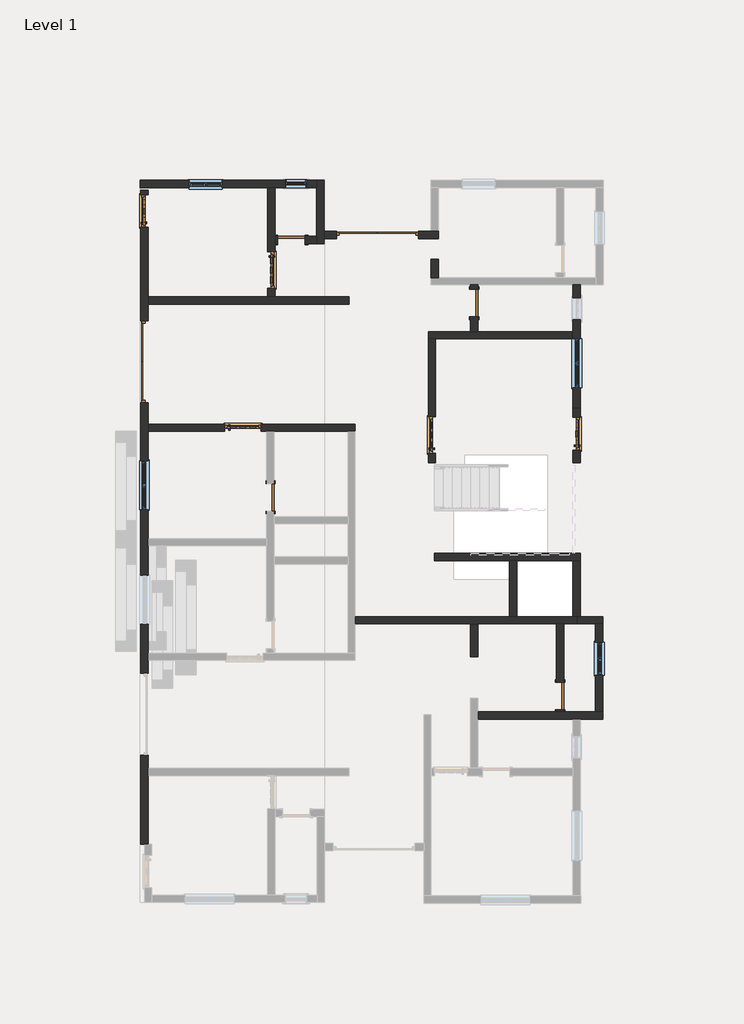
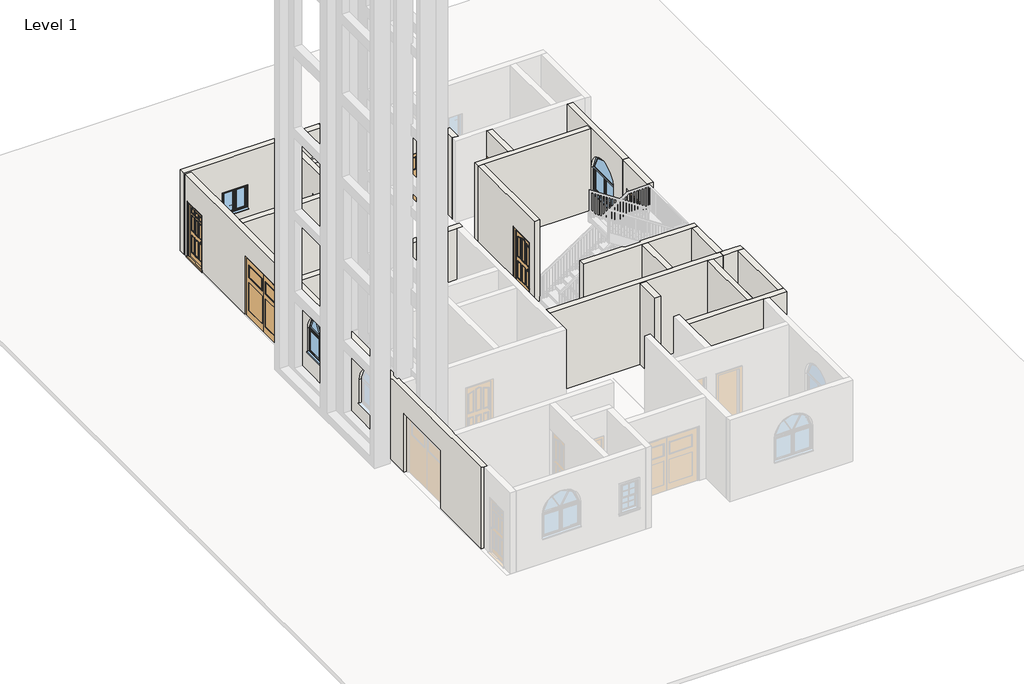
# One storey, part 2 of 4: 23 walls, 11 doors, 5 windows.
"""IFC4 building model written with IfcOpenShell, lengths in millimetres."""

from ifc_helpers import new_model, si_unit, point, frame, frame_2d, origin, origin_with_axes, place, context, project, spatial, polyline, circle_curve, trimmed, segment, composite_curve, outline, extrude, faceted_brep, transform, mapped, element, save
from ifc_brep_helpers import plane_surface, revolved_surface, advanced_brep
from components import doors_extsgl_5_910x2110mm_99758a98, doors_extsgl_5_910x2110mm_d3ca6061, doors_extsgl_6_1010x2110mm_b93c615f, doors_extsgl_6_1010x2110mm_efbaf1af, doors_garage_timber_side_hung_glazing_2270x2050mm_ae99176d, doors_garage_timber_side_hung_glazing_2270x2200mm_badb7014, door_fadea3f2, door_53b1b562, window_679d2811, windows_arched_1360x910mm_c5754810, windows_dbl_w_glazing_bars_910x910mm_41eba874

model = new_model("IFC4")

# Units and contexts
model_context = context("Model", 3, world=origin())
ifc_project = project(units=[si_unit("LENGTHUNIT", "METRE", prefix="MILLI")], contexts=[model_context])

# Site, building, storey
site = spatial("IfcSite", under=ifc_project)
building = spatial("IfcBuilding", under=site)
storey = spatial("IfcBuildingStorey", under=building, Name="Level 1", Elevation=0.0)

# Doors
placement = place(None, origin())
doors_extsgl_5_910x2110mm_shape = doors_extsgl_5_910x2110mm_99758a98(model_context)
element("IfcDoor", 1, ObjectType="Doors_ExtSgl_5 : 910x2110mm", at=placement, inside=storey, context=model_context, shape_type="MappedRepresentation", body=[
    mapped(doors_extsgl_5_910x2110mm_shape, transform((5761.5890963, 2376.5107951, 0.0), x_axis=(0.0, 1.0, 0.0), y_axis=(-1.0, 0.0, 0.0), z_axis=(0.0, 0.0, 1.0))),
])
doors_extsgl_5_910x2110mm_2_shape = doors_extsgl_5_910x2110mm_d3ca6061(model_context)
element("IfcDoor", 2, ObjectType="Doors_ExtSgl_5 : 910x2110mm", at=placement, inside=storey, context=model_context, shape_type="MappedRepresentation", body=[
    mapped(doors_extsgl_5_910x2110mm_2_shape, transform((-6229.2013636, 8553.74399, 0.0), x_axis=(0.0, 1.0, 0.0), y_axis=(-1.0, 0.0, 0.0), z_axis=(0.0, 0.0, 1.0))),
])
doors_extsgl_6_1010x2110mm_shape = doors_extsgl_6_1010x2110mm_b93c615f(model_context)
doors_extsgl_6_1010x2110mm_2_shape = doors_extsgl_6_1010x2110mm_efbaf1af(model_context)
element("IfcDoor", 3, ObjectType="Doors_ExtSgl_6 : 1010x2110mm", at=placement, inside=storey, context=model_context, shape_type="MappedRepresentation", body=[
    mapped(doors_extsgl_6_1010x2110mm_shape, transform((-2709.3109037, 6913.1295584, 0.0), x_axis=(0.0, -1.0, 0.0), y_axis=(1.0, 0.0, 0.0), z_axis=(0.0, 0.0, 1.0))),
    mapped(doors_extsgl_6_1010x2110mm_2_shape, transform((-2709.3109037, 6913.1295584, 0.0), x_axis=(0.0, -1.0, 0.0), y_axis=(1.0, 0.0, 0.0), z_axis=(0.0, 0.0, 1.0))),
])
element("IfcDoor", 4, ObjectType="Doors_ExtSgl_6 : 1010x2110mm", at=placement, inside=storey, context=model_context, shape_type="MappedRepresentation", body=[
    mapped(doors_extsgl_6_1010x2110mm_shape, transform((1748.3890963, 2341.0628918, 0.0), x_axis=(0.0, 1.0, 0.0), y_axis=(-1.0, 0.0, 0.0), z_axis=(0.0, 0.0, 1.0))),
    mapped(doors_extsgl_6_1010x2110mm_2_shape, transform((1748.3890963, 2341.0628918, 0.0), x_axis=(0.0, 1.0, 0.0), y_axis=(-1.0, 0.0, 0.0), z_axis=(0.0, 0.0, 1.0))),
])
element("IfcDoor", 5, ObjectType="Doors_ExtSgl_6 : 1010x2110mm", at=placement, inside=storey, context=model_context, shape_type="MappedRepresentation", body=[
    mapped(doors_extsgl_6_1010x2110mm_shape, transform((-3496.7442371, 2544.2962251, 0.0), x_axis=(1.0, 0.0, 0.0), y_axis=(0.0, 1.0, 0.0), z_axis=(0.0, 0.0, 1.0))),
    mapped(doors_extsgl_6_1010x2110mm_2_shape, transform((-3496.7442371, 2544.2962251, 0.0), x_axis=(1.0, 0.0, 0.0), y_axis=(0.0, 1.0, 0.0), z_axis=(0.0, 0.0, 1.0))),
])
doors_garage_timber_side_hung_glazing_2270x2050mm_shape = doors_garage_timber_side_hung_glazing_2270x2050mm_ae99176d(model_context)
element("IfcDoor", 6, ObjectType="Doors_Garage_Timber_Side_Hung_Glazing : 2270x2050mm", at=placement, inside=storey, context=model_context, shape_type="MappedRepresentation", body=[
    mapped(doors_garage_timber_side_hung_glazing_2270x2050mm_shape, transform((237.0890963, 7890.9962251, 0.0), x_axis=(1.0, 0.0, 0.0), y_axis=(0.0, 1.0, 0.0), z_axis=(0.0, 0.0, 1.0))),
])
doors_garage_timber_side_hung_glazing_2270x2200mm_shape = doors_garage_timber_side_hung_glazing_2270x2200mm_badb7014(model_context)
element("IfcDoor", 7, ObjectType="Doors_Garage_Timber_Side_Hung_Glazing : 2270x2200mm", at=placement, inside=storey, context=model_context, shape_type="MappedRepresentation", body=[
    mapped(doors_garage_timber_side_hung_glazing_2270x2200mm_shape, transform((-6229.2013636, 4373.0962251, 0.0), x_axis=(0.0, -1.0, 0.0), y_axis=(1.0, 0.0, 0.0), z_axis=(0.0, 0.0, 1.0))),
])
door_shape = door_fadea3f2(model_context)
element("IfcDoor", 8, ObjectType="Single-Flush : 30\" x 80\"", at=placement, inside=storey, context=model_context, shape_type="MappedRepresentation", body=[
    mapped(door_shape, transform((5304.3890963, -4897.9037749, 0.0), x_axis=(0.0, -1.0, 0.0), y_axis=(1.0, 0.0, 0.0), z_axis=(0.0, 0.0, 1.0))),
])
door_2_shape = door_53b1b562(model_context)
element("IfcDoor", 9, ObjectType="Single-Flush : 30\" x 80\"", at=placement, inside=storey, context=model_context, shape_type="MappedRepresentation", body=[
    mapped(door_2_shape, transform((-2150.5109037, 7751.2962251, 0.0), x_axis=(-1.0, 0.0, 0.0), y_axis=(0.0, -1.0, 0.0), z_axis=(0.0, 0.0, 1.0))),
])
element("IfcDoor", 10, ObjectType="Single-Flush : 30\" x 80\"", at=placement, inside=storey, context=model_context, shape_type="MappedRepresentation", body=[
    mapped(door_2_shape, transform((2916.7890963, 5998.6962251, 0.0), x_axis=(0.0, 1.0, 0.0), y_axis=(-1.0, 0.0, 0.0), z_axis=(0.0, 0.0, 1.0))),
])
element("IfcDoor", 11, ObjectType="Single-Flush : 30\" x 80\"", at=placement, inside=storey, context=model_context, shape_type="MappedRepresentation", body=[
    mapped(door_2_shape, transform((-2734.7109037, 613.8962251, 0.0), x_axis=(0.0, 1.0, 0.0), y_axis=(-1.0, 0.0, 0.0), z_axis=(0.0, 0.0, 1.0))),
])

# Walls
element("IfcWall", 12, ObjectType="Generic - 9\" w", at=placement, inside=storey, context=model_context, shape_type="SweptSolid", body=[
    extrude(outline(polyline([(6506.6962251, 0.0), (3087.7441284, 0.0), (3087.7441284, 3048.0), (6506.6962251, 3048.0), (6506.6962251, 0.0)]), holes=[polyline([(6151.0962251, 1981.2), (5541.4962251, 1981.2), (5541.4962251, 914.4), (6151.0962251, 914.4), (6151.0962251, 1981.2)]), composite_curve([segment(polyline([(5016.7786331, 685.6617803), (5016.7786331, 1595.6617803)]), True, "CONTINUOUS"), segment(trimmed(circle_curve(frame_2d((4336.7786331, 1595.6617803)), 680.0), [point((5016.7786331, 1595.6617803))], [point((3656.7786331, 1595.6617803))], True, "CARTESIAN"), True, "CONTINUOUS"), segment(polyline([(3656.7786331, 1595.6617803), (3656.7786331, 685.6617803), (5016.7786331, 685.6617803)]), True, "CONTINUOUS")], self_intersect=False)]), frame((5659.9890963, 0.0, 0.0), z_axis=(1.0, 0.0, 0.0), x_axis=(0.0, 1.0, 0.0)), (0.0, 0.0, 1.0), 203.2),
])
element("IfcWall", 13, ObjectType="Generic - 9\" w", at=placement, inside=storey, context=model_context, shape_type="Brep", body=[
    faceted_brep([(6485.4890963, -2688.1037749, 0.0), (5863.1890963, -2688.1037749, 0.0), (5761.5890963, -2688.1037749, 0.0), (5761.5890963, -2688.1037749, 3048.0), (5863.1890963, -2688.1037749, 3048.0), (6485.4890963, -2688.1037749, 3048.0), (6485.4890963, -2891.3037749, 0.0), (6485.4890963, -2891.3037749, 3048.0), (6282.2890963, -2891.3037749, 3048.0), (5761.5890963, -2891.3037749, 3048.0), (5761.5890963, -2891.3037749, 0.0), (6282.2890963, -2891.3037749, 0.0)], [[[0, 1, 2, 3, 4, 5]], [[6, 7, 8, 9, 10, 11]], [[2, 1, 0, 6, 11, 10]], [[3, 2, 10, 9]], [[5, 4, 3, 9, 8, 7]], [[0, 5, 7, 6]]]),
])
element("IfcWall", 14, ObjectType="Generic - 9\" w", at=placement, inside=storey, context=model_context, shape_type="Brep", body=[
    faceted_brep([(5761.5890963, -2688.1037749, 0.0), (5659.9890963, -2688.1037749, 0.0), (4097.8890963, -2688.1037749, 0.0), (3894.6890963, -2688.1037749, 0.0), (-385.2109037, -2688.1037749, 0.0), (-385.2109037, -2688.1037749, 3048.0), (3894.6890963, -2688.1037749, 3048.0), (4097.8890963, -2688.1037749, 3048.0), (5659.9890963, -2688.1037749, 3048.0), (5761.5890963, -2688.1037749, 3048.0), (5761.5890963, -2891.3037749, 0.0), (5761.5890963, -2891.3037749, 3048.0), (5405.9890963, -2891.3037749, 3048.0), (5202.7890963, -2891.3037749, 3048.0), (-385.2109037, -2891.3037749, 3048.0), (-385.2109037, -2891.3037749, 0.0), (5202.7890963, -2891.3037749, 0.0), (5405.9890963, -2891.3037749, 0.0)], [[[0, 1, 2, 3, 4, 5, 6, 7, 8, 9]], [[10, 11, 12, 13, 14, 15, 16, 17]], [[4, 3, 2, 1, 0, 10, 17, 16, 15]], [[9, 8, 7, 6, 5, 14, 13, 12, 11]], [[0, 9, 11, 10]], [[5, 4, 15, 14]]]),
])
element("IfcWall", 15, ObjectType="Generic - 9\" w", at=placement, inside=storey, context=model_context, shape_type="SweptSolid", body=[
    extrude(outline(polyline([(3894.6890963, -2688.1037749), (3894.6890963, -1138.7037749), (4097.8890963, -1138.7037749), (4097.8890963, -2688.1037749), (3894.6890963, -2688.1037749)])), origin_with_axes(), (0.0, 0.0, 1.0), 3048.0),
])
element("IfcWall", 16, ObjectType="Generic - 9\" w", at=placement, inside=storey, context=model_context, shape_type="Brep", body=[
    faceted_brep([(5863.1890963, -935.5037749, 0.0), (1812.4805171, -935.5037749, 0.0), (1812.4805171, -935.5037749, 3048.0), (5863.1890963, -935.5037749, 3048.0), (5863.1890963, -1138.7037749, 0.0), (5863.1890963, -1138.7037749, 3048.0), (5659.9890963, -1138.7037749, 3048.0), (4097.8890963, -1138.7037749, 3048.0), (3894.6890963, -1138.7037749, 3048.0), (1812.4805171, -1138.7037749, 3048.0), (1812.4805171, -1138.7037749, 0.0), (3894.6890963, -1138.7037749, 0.0), (4097.8890963, -1138.7037749, 0.0), (5659.9890963, -1138.7037749, 0.0)], [[[0, 1, 2, 3]], [[4, 5, 6, 7, 8, 9, 10, 11, 12, 13]], [[1, 0, 4, 13, 12, 11, 10]], [[2, 1, 10, 9]], [[3, 2, 9, 8, 7, 6, 5]], [[0, 3, 5, 4]]]),
])
element("IfcWall", 17, ObjectType="Generic - 9\" w", at=placement, inside=storey, context=model_context, shape_type="Brep", body=[
    faceted_brep([(5659.9890963, -1138.7037749, 0.0), (5659.9890963, -2688.1037749, 0.0), (5659.9890963, -2688.1037749, 3048.0), (5659.9890963, -1138.7037749, 3048.0), (5863.1890963, -1138.7037749, 0.0), (5863.1890963, -1138.7037749, 3048.0), (5863.1890963, -2688.1037749, 3048.0), (5863.1890963, -2688.1037749, 0.0), (5761.5890963, -2688.1037749, 0.0), (5761.5890963, -2688.1037749, 3048.0)], [[[0, 1, 2, 3]], [[4, 5, 6, 7]], [[1, 0, 4, 7, 8]], [[3, 2, 9, 6, 5]], [[2, 1, 8, 7, 6, 9]], [[0, 3, 5, 4]]]),
])
element("IfcWall", 18, ObjectType="Generic - 9\" w", at=placement, inside=storey, context=model_context, shape_type="AdvancedBrep", body=[
    advanced_brep(
    [(-6330.8013636, 3238.0962251, 0.0), (-6330.8013636, -4267.1251987, 0.0), (-6330.8013636, -4267.1251987, 2200.0), (-6330.8013636, -6537.1251987, 2200.0), (-6330.8013636, -6537.1251987, 0.0), (-6330.8013636, -9007.7845215, 0.0), (-6330.8013636, -9007.7845215, 3048.0), (-6330.8013636, 9129.8816143, 3048.0), (-6330.8013636, 9129.8816143, 0.0), (-6330.8013636, 9008.7773233, 0.0), (-6330.8013636, 9008.7773233, 2110.0), (-6330.8013636, 8098.7773233, 2110.0), (-6330.8013636, 8098.7773233, 0.0), (-6330.8013636, 5508.0962251, 0.0), (-6330.8013636, 5508.0962251, 2200.0), (-6330.8013636, 3238.0962251, 2200.0), (-6330.8013636, 276.7962251, 914.4), (-6330.8013636, 1636.7962251, 914.4), (-6330.8013636, 1636.7962251, 1824.4), (-6330.8013636, 276.7962251, 1824.4), (-6330.8013636, -1538.2037749, 914.4), (-6330.8013636, -1538.2037749, 1824.4), (-6330.8013636, -2898.2037749, 1824.4), (-6330.8013636, -2898.2037749, 914.4), (-6127.6013636, -4267.1251987, 2200.0), (-6127.6013636, -4267.1251987, 0.0), (-6127.6013636, -3907.3037749, 0.0), (-6127.6013636, -3704.1037749, 0.0), (-6127.6013636, -732.3037749, 0.0), (-6127.6013636, -529.1037749, 0.0), (-6127.6013636, 2442.6962251, 0.0), (-6127.6013636, 2645.8962251, 0.0), (-6127.6013636, 3238.0962251, 0.0), (-6127.6013636, 3238.0962251, 2200.0), (-6127.6013636, 5508.0962251, 2200.0), (-6127.6013636, 5508.0962251, 0.0), (-6127.6013636, 5973.2962251, 0.0), (-6127.6013636, 6176.4962251, 0.0), (-6127.6013636, 8098.7773233, 0.0), (-6127.6013636, 8098.7773233, 2110.0), (-6127.6013636, 9008.7773233, 2110.0), (-6127.6013636, 9008.7773233, 0.0), (-6127.6013636, 9129.8816143, 0.0), (-6127.6013636, 9129.8816143, 3048.0), (-6127.6013636, 6176.4962251, 3048.0), (-6127.6013636, 5973.2962251, 3048.0), (-6127.6013636, 2645.8962251, 3048.0), (-6127.6013636, 2442.6962251, 3048.0), (-6127.6013636, -529.1037749, 3048.0), (-6127.6013636, -732.3037749, 3048.0), (-6127.6013636, -3704.1037749, 3048.0), (-6127.6013636, -3907.3037749, 3048.0), (-6127.6013636, -6896.9466225, 3048.0), (-6127.6013636, -7100.1466225, 3048.0), (-6127.6013636, -9007.7845215, 3048.0), (-6127.6013636, -9007.7845215, 0.0), (-6127.6013636, -7100.1466225, 0.0), (-6127.6013636, -6896.9466225, 0.0), (-6127.6013636, -6537.1251987, 0.0), (-6127.6013636, -6537.1251987, 2200.0), (-6127.6013636, 276.7962251, 914.4), (-6127.6013636, 276.7962251, 1824.4), (-6127.6013636, 1636.7962251, 1824.4), (-6127.6013636, 1636.7962251, 914.4), (-6127.6013636, -1538.2037749, 914.4), (-6127.6013636, -2898.2037749, 914.4), (-6127.6013636, -2898.2037749, 1824.4), (-6127.6013636, -1538.2037749, 1824.4), (-6229.2013636, -9007.7845215, 0.0), (-6229.2013636, -9007.7845215, 3048.0)],
    [
        (0, 1),
        (1, 2),
        (2, 3),
        (3, 4),
        (4, 5),
        (5, 6),
        (6, 7),
        (7, 8),
        (8, 9),
        (9, 10),
        (10, 11),
        (11, 12),
        (12, 13),
        (13, 14),
        (14, 15),
        (15, 0),
        (16, 17),
        (17, 18),
        (18, 19, circle_curve(frame((-6330.8013636, 956.7962251, 1824.4), z_axis=(1.0, 0.0, 0.0), x_axis=(0.0, 1.0, 0.0)), 680.0)),
        (19, 16),
        (20, 21),
        (21, 22, circle_curve(frame((-6330.8013636, -2218.2037749, 1824.4), z_axis=(1.0, 0.0, 0.0), x_axis=(0.0, -1.0, 0.0)), 680.0)),
        (22, 23),
        (23, 20),
        (24, 25),
        (25, 26),
        (26, 27),
        (27, 28),
        (28, 29),
        (29, 30),
        (30, 31),
        (31, 32),
        (32, 33),
        (33, 34),
        (34, 35),
        (35, 36),
        (36, 37),
        (37, 38),
        (38, 39),
        (39, 40),
        (40, 41),
        (41, 42),
        (42, 43),
        (43, 44),
        (44, 45),
        (45, 46),
        (46, 47),
        (47, 48),
        (48, 49),
        (49, 50),
        (50, 51),
        (51, 52),
        (52, 53),
        (53, 54),
        (54, 55),
        (55, 56),
        (56, 57),
        (57, 58),
        (58, 59),
        (59, 24),
        (60, 61),
        (61, 62, circle_curve(frame((-6127.6013636, 956.7962251, 1824.4), z_axis=(-1.0, 0.0, 0.0), x_axis=(0.0, 1.0, 0.0)), 680.0)),
        (62, 63),
        (63, 60),
        (64, 65),
        (65, 66),
        (66, 67, circle_curve(frame((-6127.6013636, -2218.2037749, 1824.4), z_axis=(-1.0, 0.0, 0.0), x_axis=(0.0, -1.0, 0.0)), 680.0)),
        (67, 64),
        (41, 9),
        (8, 42),
        (12, 38),
        (35, 13),
        (55, 68),
        (68, 5),
        (4, 58),
        (25, 1),
        (0, 32),
        (54, 69),
        (69, 6),
        (43, 7),
        (11, 39),
        (40, 10),
        (34, 14),
        (15, 33),
        (3, 59),
        (24, 2),
        (60, 16),
        (19, 61),
        (18, 62),
        (17, 63),
        (20, 64),
        (67, 21),
        (66, 22),
        (65, 23),
    ],
    [
        plane_surface(frame((-6330.8013636, 2442.6962251, 0.0), z_axis=(-1.0, 0.0, 0.0), x_axis=(0.0, -1.0, 0.0))),
        plane_surface(frame((-6127.6013636, 2442.6962251, 0.0), z_axis=(1.0, 0.0, 0.0), x_axis=(0.0, 1.0, 0.0))),
        plane_surface(frame((-6330.8013636, 9129.8816143, 0.0), z_axis=(0.0, 0.0, -1.0), x_axis=(1.0, 0.0, 0.0))),
        plane_surface(frame((-6330.8013636, -9007.7845215, 0.0), z_axis=(0.0, -1.0, 0.0), x_axis=(1.0, 0.0, 0.0))),
        plane_surface(frame((-6330.8013636, -9007.7845215, 3048.0), z_axis=(0.0, 0.0, 1.0), x_axis=(1.0, 0.0, 0.0))),
        plane_surface(frame((-6330.8013636, 9129.8816143, 3048.0), z_axis=(0.0, 1.0, 0.0), x_axis=(1.0, 0.0, 0.0))),
        plane_surface(frame((-6330.8013636, 8098.7773233, 2110.0), z_axis=(0.0, 1.0, 0.0), x_axis=(1.0, 0.0, 0.0))),
        plane_surface(frame((-6330.8013636, 9008.7773233, 0.0), z_axis=(0.0, -1.0, 0.0), x_axis=(1.0, 0.0, 0.0))),
        plane_surface(frame((-6330.8013636, 9008.7773233, 2110.0), z_axis=(0.0, 0.0, -1.0), x_axis=(1.0, 0.0, 0.0))),
        plane_surface(frame((-6127.6013636, 5508.0962251, 2200.0), z_axis=(0.0, -1.0, 0.0), x_axis=(-1.0, 0.0, 0.0))),
        plane_surface(frame((-6127.6013636, 3238.0962251, 0.0), z_axis=(0.0, 1.0, 0.0), x_axis=(-1.0, 0.0, 0.0))),
        plane_surface(frame((-6127.6013636, 3238.0962251, 2200.0), z_axis=(0.0, 0.0, -1.0), x_axis=(-1.0, 0.0, 0.0))),
        plane_surface(frame((-6330.8013636, -6537.1251987, 2200.0), z_axis=(0.0, 1.0, 0.0), x_axis=(1.0, 0.0, 0.0))),
        plane_surface(frame((-6330.8013636, -4267.1251987, 0.0), z_axis=(0.0, -1.0, 0.0), x_axis=(1.0, 0.0, 0.0))),
        plane_surface(frame((-6330.8013636, -4267.1251987, 2200.0), z_axis=(0.0, 0.0, -1.0), x_axis=(1.0, 0.0, 0.0))),
        plane_surface(frame((-6127.6013636, 276.7962251, 914.4), z_axis=(0.0, 1.0, 0.0), x_axis=(-1.0, 0.0, 0.0))),
        revolved_surface(polyline([(-6330.8013636, 1636.7962251, 1824.4), (-6127.6013636, 1636.7962251, 1824.4)]), (-6127.6013636, 956.7962251, 1824.4), (-1.0, 0.0, 0.0)),
        plane_surface(frame((-6127.6013636, 1636.7962251, 1824.4), z_axis=(0.0, -1.0, 0.0), x_axis=(-1.0, 0.0, 0.0))),
        plane_surface(frame((-6127.6013636, 1636.7962251, 914.4), z_axis=(0.0, 0.0, 1.0), x_axis=(-1.0, 0.0, 0.0))),
        plane_surface(frame((-6330.8013636, -1538.2037749, 914.4), z_axis=(0.0, -1.0, 0.0), x_axis=(1.0, 0.0, 0.0))),
        revolved_surface(polyline([(-6127.6013636, -2898.2037749, 1824.4), (-6330.8013636, -2898.2037749, 1824.4)]), (-6330.8013636, -2218.2037749, 1824.4), (1.0, 0.0, 0.0)),
        plane_surface(frame((-6330.8013636, -2898.2037749, 1824.4), z_axis=(0.0, 1.0, 0.0), x_axis=(1.0, 0.0, 0.0))),
        plane_surface(frame((-6330.8013636, -2898.2037749, 914.4), z_axis=(0.0, 0.0, 1.0), x_axis=(1.0, 0.0, 0.0))),
    ],
    [
        (0, [[1, 2, 3, 4, 5, 6, 7, 8, 9, 10, 11, 12, 13, 14, 15, 16], [17, 18, 19, 20], [21, 22, 23, 24]]),
        (1, [[25, 26, 27, 28, 29, 30, 31, 32, 33, 34, 35, 36, 37, 38, 39, 40, 41, 42, 43, 44, 45, 46, 47, 48, 49, 50, 51, 52, 53, 54, 55, 56, 57, 58, 59, 60], [61, 62, 63, 64], [65, 66, 67, 68]]),
        (2, [[-42, 69, -9, 70]]),
        (2, [[-13, 71, -38, -37, -36, 72]]),
        (2, [[-58, -57, -56, 73, 74, -5, 75]]),
        (2, [[-32, -31, -30, -29, -28, -27, -26, 76, -1, 77]]),
        (3, [[-6, -74, -73, -55, 78, 79]]),
        (4, [[-7, -79, -78, -54, -53, -52, -51, -50, -49, -48, -47, -46, -45, -44, 80]]),
        (5, [[-8, -80, -43, -70]]),
        (6, [[-12, 81, -39, -71]]),
        (7, [[-10, -69, -41, 82]]),
        (8, [[-11, -82, -40, -81]]),
        (9, [[-35, 83, -14, -72]]),
        (10, [[-33, -77, -16, 84]]),
        (11, [[-34, -84, -15, -83]]),
        (12, [[-4, 85, -59, -75]]),
        (13, [[-2, -76, -25, 86]]),
        (14, [[-3, -86, -60, -85]]),
        (15, [[-61, 87, -20, 88]]),
        (16, [[-62, -88, -19, 89]]),
        (17, [[-63, -89, -18, 90]]),
        (18, [[-64, -90, -17, -87]]),
        (19, [[-21, 91, -68, 92]]),
        (20, [[-22, -92, -67, 93]]),
        (21, [[-23, -93, -66, 94]]),
        (22, [[-24, -94, -65, -91]]),
    ],
),
])
element("IfcWall", 19, ObjectType="Generic - 9\" w", at=placement, inside=storey, context=model_context, shape_type="SweptSolid", body=[
    extrude(outline(polyline([(3087.7441284, 0.0), (2831.5441284, 0.0), (2831.5441284, 2110.0), (1921.5441284, 2110.0), (1921.5441284, 0.0), (1579.0962251, 0.0), (1579.0962251, 3048.0), (3087.7441284, 3048.0), (3087.7441284, 0.0)])), frame((5659.9890963, 0.0, 0.0), z_axis=(1.0, 0.0, 0.0), x_axis=(0.0, 1.0, 0.0)), (0.0, 0.0, 1.0), 203.2),
])
element("IfcWall", 20, ObjectType="Generic - 9\" w", at=placement, inside=storey, context=model_context, shape_type="Brep", body=[
    faceted_brep([(-1452.0109037, 9401.8527313, 0.0), (-6354.2109037, 9401.8527313, 0.0), (-6354.2109037, 9401.8527313, 3048.0), (-1452.0109037, 9401.8527313, 3048.0), (-4076.7609037, 9401.8527313, 1824.4), (-4986.7609037, 9401.8527313, 1824.4), (-4986.7609037, 9401.8527313, 914.4), (-4076.7609037, 9401.8527313, 914.4), (-2334.6609037, 9401.8527313, 1981.2), (-2334.6609037, 9401.8527313, 914.4), (-1725.0609037, 9401.8527313, 914.4), (-1725.0609037, 9401.8527313, 1981.2), (-1452.0109037, 9198.6527313, 0.0), (-1452.0109037, 9198.6527313, 3048.0), (-2607.7109037, 9198.6527313, 3048.0), (-2810.9109037, 9198.6527313, 3048.0), (-6354.2109037, 9198.6527313, 3048.0), (-6354.2109037, 9198.6527313, 0.0), (-2810.9109037, 9198.6527313, 0.0), (-2607.7109037, 9198.6527313, 0.0), (-4076.7609037, 9198.6527313, 1824.4), (-4076.7609037, 9198.6527313, 914.4), (-4986.7609037, 9198.6527313, 914.4), (-4986.7609037, 9198.6527313, 1824.4), (-2334.6609037, 9198.6527313, 1981.2), (-1725.0609037, 9198.6527313, 1981.2), (-1725.0609037, 9198.6527313, 914.4), (-2334.6609037, 9198.6527313, 914.4)], [[[0, 1, 2, 3], [4, 5, 6, 7], [8, 9, 10, 11]], [[12, 13, 14, 15, 16, 17, 18, 19], [20, 21, 22, 23], [24, 25, 26, 27]], [[1, 0, 12, 19, 18, 17]], [[2, 1, 17, 16]], [[3, 2, 16, 15, 14, 13]], [[0, 3, 13, 12]], [[21, 20, 4, 7]], [[22, 21, 7, 6]], [[23, 22, 6, 5]], [[20, 23, 5, 4]], [[9, 8, 24, 27]], [[10, 9, 27, 26]], [[11, 10, 26, 25]], [[8, 11, 25, 24]]]),
])
element("IfcWall", 21, ObjectType="Generic -4.5\" p", at=placement, inside=storey, context=model_context, shape_type="Brep", body=[
    faceted_brep([(-2810.9109037, 6408.0962251, 2110.0), (-2810.9109037, 6408.0962251, 0.0), (-2810.9109037, 6176.4962251, 0.0), (-2810.9109037, 6176.4962251, 3048.0), (-2810.9109037, 9198.6527313, 3048.0), (-2810.9109037, 9198.6527313, 0.0), (-2810.9109037, 7418.0962251, 0.0), (-2810.9109037, 7418.0962251, 2110.0), (-2607.7109037, 6176.4962251, 0.0), (-2607.7109037, 6408.0962251, 0.0), (-2607.7109037, 6408.0962251, 2110.0), (-2607.7109037, 7418.0962251, 2110.0), (-2607.7109037, 7418.0962251, 0.0), (-2607.7109037, 7649.6962251, 0.0), (-2607.7109037, 7852.8962251, 0.0), (-2607.7109037, 9198.6527313, 0.0), (-2607.7109037, 9198.6527313, 3048.0), (-2607.7109037, 7852.8962251, 3048.0), (-2607.7109037, 7649.6962251, 3048.0), (-2607.7109037, 6176.4962251, 3048.0)], [[[0, 1, 2, 3, 4, 5, 6, 7]], [[8, 9, 10, 11, 12, 13, 14, 15, 16, 17, 18, 19]], [[6, 5, 15, 14, 13, 12]], [[2, 1, 9, 8]], [[4, 3, 19, 18, 17, 16]], [[3, 2, 8, 19]], [[12, 11, 7, 6]], [[10, 9, 1, 0]], [[11, 10, 0, 7]], [[5, 4, 16, 15]]]),
])
element("IfcWall", 22, ObjectType="Generic -4.5\" p", at=placement, inside=storey, context=model_context, shape_type="Brep", body=[
    faceted_brep([(-6127.6013636, 5973.2962251, 0.0), (-550.3109037, 5973.2962251, 0.0), (-550.3109037, 5973.2962251, 3048.0), (-6127.6013636, 5973.2962251, 3048.0), (-6127.6013636, 6176.4962251, 0.0), (-6127.6013636, 6176.4962251, 3048.0), (-2810.9109037, 6176.4962251, 3048.0), (-2607.7109037, 6176.4962251, 3048.0), (-550.3109037, 6176.4962251, 3048.0), (-550.3109037, 6176.4962251, 0.0), (-2607.7109037, 6176.4962251, 0.0), (-2810.9109037, 6176.4962251, 0.0)], [[[0, 1, 2, 3]], [[4, 5, 6, 7, 8, 9, 10, 11]], [[1, 0, 4, 11, 10, 9]], [[2, 1, 9, 8]], [[3, 2, 8, 7, 6, 5]], [[0, 3, 5, 4]]]),
])
element("IfcWall", 23, ObjectType="Generic -4.5\" p", at=placement, inside=storey, context=model_context, shape_type="Brep", body=[
    faceted_brep([(-1452.0109037, 9401.8527313, 0.0), (-1452.0109037, 9198.6527313, 0.0), (-1452.0109037, 7852.8962251, 0.0), (-1452.0109037, 7649.6962251, 0.0), (-1452.0109037, 7649.6962251, 3048.0), (-1452.0109037, 7852.8962251, 3048.0), (-1452.0109037, 9198.6527313, 3048.0), (-1452.0109037, 9401.8527313, 3048.0), (-1248.8109037, 9401.8527313, 0.0), (-1248.8109037, 9401.8527313, 3048.0), (-1248.8109037, 7992.5962251, 3048.0), (-1248.8109037, 7789.3962251, 3048.0), (-1248.8109037, 7649.6962251, 3048.0), (-1248.8109037, 7649.6962251, 0.0), (-1248.8109037, 7789.3962251, 0.0), (-1248.8109037, 7992.5962251, 0.0)], [[[0, 1, 2, 3, 4, 5, 6, 7]], [[8, 9, 10, 11, 12, 13, 14, 15]], [[3, 2, 1, 0, 8, 15, 14, 13]], [[7, 6, 5, 4, 12, 11, 10, 9]], [[4, 3, 13, 12]], [[0, 7, 9, 8]]]),
])
element("IfcWall", 24, ObjectType="Generic -4.5\" p", at=placement, inside=storey, context=model_context, shape_type="SweptSolid", body=[
    extrude(outline(polyline([(0.0, -2607.7109037), (0.0, -2531.5109037), (2032.0, -2531.5109037), (2032.0, -1769.5109037), (0.0, -1769.5109037), (0.0, -1452.0109037), (3048.0, -1452.0109037), (3048.0, -2607.7109037), (0.0, -2607.7109037)])), frame((0.0, 7649.6962251, 0.0), z_axis=(0.0, 1.0, 0.0), x_axis=(0.0, 0.0, 1.0)), (0.0, 0.0, 1.0), 203.2),
])
element("IfcWall", 25, ObjectType="Generic -4.5\" p", at=placement, inside=storey, context=model_context, shape_type="Brep", body=[
    faceted_brep([(1372.0890963, 7789.3962251, 2050.0), (1372.0890963, 7789.3962251, 0.0), (1926.1890963, 7789.3962251, 0.0), (1926.1890963, 7789.3962251, 3048.0), (-1248.8109037, 7789.3962251, 3048.0), (-1248.8109037, 7789.3962251, 0.0), (-897.9109037, 7789.3962251, 0.0), (-897.9109037, 7789.3962251, 2050.0), (1926.1890963, 7992.5962251, 0.0), (1722.9890963, 7992.5962251, 0.0), (1372.0890963, 7992.5962251, 0.0), (1372.0890963, 7992.5962251, 2050.0), (-897.9109037, 7992.5962251, 2050.0), (-897.9109037, 7992.5962251, 0.0), (-1248.8109037, 7992.5962251, 0.0), (-1248.8109037, 7992.5962251, 3048.0), (1722.9890963, 7992.5962251, 3048.0), (1926.1890963, 7992.5962251, 3048.0)], [[[0, 1, 2, 3, 4, 5, 6, 7]], [[8, 9, 10, 11, 12, 13, 14, 15, 16, 17]], [[6, 5, 14, 13]], [[2, 1, 10, 9, 8]], [[4, 3, 17, 16, 15]], [[5, 4, 15, 14]], [[3, 2, 8, 17]], [[13, 12, 7, 6]], [[11, 10, 1, 0]], [[12, 11, 0, 7]]]),
])
element("IfcWall", 26, ObjectType="Generic -4.5\" p", at=placement, inside=storey, context=model_context, shape_type="SweptSolid", body=[
    extrude(outline(polyline([(1926.1890963, 7221.6524875), (1926.1890963, 6709.8962251), (1722.9890963, 6709.8962251), (1722.9890963, 7221.6524875), (1926.1890963, 7221.6524875)])), origin_with_axes(), (0.0, 0.0, 1.0), 3048.0),
])
element("IfcWall", 27, ObjectType="Generic -4.5\" p", at=placement, inside=storey, context=model_context, shape_type="SweptSolid", body=[
    extrude(outline(polyline([(6506.6962251, 0.0), (6379.6962251, 0.0), (6379.6962251, 2032.0), (5617.6962251, 2032.0), (5617.6962251, 0.0), (5211.2962251, 0.0), (5211.2962251, 3048.0), (6506.6962251, 3048.0), (6506.6962251, 0.0)])), frame((2815.1890963, 0.0, 0.0), z_axis=(1.0, 0.0, 0.0), x_axis=(0.0, 1.0, 0.0)), (0.0, 0.0, 1.0), 203.2),
])
element("IfcWall", 28, ObjectType="Generic -4.5\" p", at=placement, inside=storey, context=model_context, shape_type="Brep", body=[
    faceted_brep([(5634.5890963, 5211.2962251, 0.0), (3018.3890963, 5211.2962251, 0.0), (2815.1890963, 5211.2962251, 0.0), (1646.7890963, 5211.2962251, 0.0), (1646.7890963, 5211.2962251, 3048.0), (2815.1890963, 5211.2962251, 3048.0), (3018.3890963, 5211.2962251, 3048.0), (5634.5890963, 5211.2962251, 3048.0), (5634.5890963, 5008.0962251, 0.0), (5634.5890963, 5008.0962251, 3048.0), (1849.9890963, 5008.0962251, 3048.0), (1646.7890963, 5008.0962251, 3048.0), (1646.7890963, 5008.0962251, 0.0), (1849.9890963, 5008.0962251, 0.0)], [[[0, 1, 2, 3, 4, 5, 6, 7]], [[8, 9, 10, 11, 12, 13]], [[3, 2, 1, 0, 8, 13, 12]], [[7, 6, 5, 4, 11, 10, 9]], [[0, 7, 9, 8]], [[4, 3, 12, 11]]]),
])
element("IfcWall", 29, ObjectType="Generic -4.5\" p", at=placement, inside=storey, context=model_context, shape_type="SweptSolid", body=[
    extrude(outline(polyline([(5008.0962251, 0.0), (2846.0962251, 0.0), (2846.0962251, 2110.0), (1836.0962251, 2110.0), (1836.0962251, 0.0), (1579.0962251, 0.0), (1579.0962251, 3048.0), (5008.0962251, 3048.0), (5008.0962251, 0.0)])), frame((1646.7890963, 0.0, 0.0), z_axis=(1.0, 0.0, 0.0), x_axis=(0.0, 1.0, 0.0)), (0.0, 0.0, 1.0), 203.2),
])
element("IfcWall", 30, ObjectType="Generic -4.5\" p", at=placement, inside=storey, context=model_context, shape_type="Brep", body=[
    faceted_brep([(-2991.7109037, 2442.6962251, 2110.0), (-2991.7109037, 2442.6962251, 0.0), (-2836.3109037, 2442.6962251, 0.0), (-2633.1109037, 2442.6962251, 0.0), (-588.4109037, 2442.6962251, 0.0), (-385.2109037, 2442.6962251, 0.0), (-385.2109037, 2442.6962251, 3048.0), (-588.4109037, 2442.6962251, 3048.0), (-2633.1109037, 2442.6962251, 3048.0), (-2836.3109037, 2442.6962251, 3048.0), (-6127.6013636, 2442.6962251, 3048.0), (-6127.6013636, 2442.6962251, 0.0), (-4001.7109037, 2442.6962251, 0.0), (-4001.7109037, 2442.6962251, 2110.0), (-385.2109037, 2645.8962251, 0.0), (-2991.7109037, 2645.8962251, 0.0), (-2991.7109037, 2645.8962251, 2110.0), (-4001.7109037, 2645.8962251, 2110.0), (-4001.7109037, 2645.8962251, 0.0), (-6127.6013636, 2645.8962251, 0.0), (-6127.6013636, 2645.8962251, 3048.0), (-385.2109037, 2645.8962251, 3048.0)], [[[0, 1, 2, 3, 4, 5, 6, 7, 8, 9, 10, 11, 12, 13]], [[14, 15, 16, 17, 18, 19, 20, 21]], [[12, 11, 19, 18]], [[5, 4, 3, 2, 1, 15, 14]], [[10, 9, 8, 7, 6, 21, 20]], [[6, 5, 14, 21]], [[18, 17, 13, 12]], [[16, 15, 1, 0]], [[17, 16, 0, 13]], [[11, 10, 20, 19]]]),
])
element("IfcWall", 31, ObjectType="Generic -4.5\" p", at=placement, inside=storey, context=model_context, shape_type="Brep", body=[
    faceted_brep([(3018.3890963, -5532.9037749, 0.0), (5659.9890963, -5532.9037749, 0.0), (5863.1890963, -5532.9037749, 0.0), (6485.4890963, -5532.9037749, 0.0), (6485.4890963, -5532.9037749, 3048.0), (5863.1890963, -5532.9037749, 3048.0), (5659.9890963, -5532.9037749, 3048.0), (3018.3890963, -5532.9037749, 3048.0), (3018.3890963, -5329.7037749, 0.0), (3018.3890963, -5329.7037749, 3048.0), (5202.7890963, -5329.7037749, 3048.0), (5405.9890963, -5329.7037749, 3048.0), (6282.2890963, -5329.7037749, 3048.0), (6485.4890963, -5329.7037749, 3048.0), (6485.4890963, -5329.7037749, 0.0), (6282.2890963, -5329.7037749, 0.0), (5405.9890963, -5329.7037749, 0.0), (5202.7890963, -5329.7037749, 0.0)], [[[0, 1, 2, 3, 4, 5, 6, 7]], [[8, 9, 10, 11, 12, 13, 14, 15, 16, 17]], [[3, 2, 1, 0, 8, 17, 16, 15, 14]], [[7, 6, 5, 4, 13, 12, 11, 10, 9]], [[0, 7, 9, 8]], [[4, 3, 14, 13]]]),
])
element("IfcWall", 32, ObjectType="Generic -4.5\" p", at=placement, inside=storey, context=model_context, shape_type="SweptSolid", body=[
    extrude(outline(polyline([(-5329.7037749, 0.0), (-5329.7037749, 3048.0), (-2891.3037749, 3048.0), (-2891.3037749, 0.0), (-5329.7037749, 0.0)]), holes=[polyline([(-3401.5037749, 1824.4), (-4311.5037749, 1824.4), (-4311.5037749, 914.4), (-3401.5037749, 914.4), (-3401.5037749, 1824.4)])]), frame((6282.2890963, 0.0, 0.0), z_axis=(1.0, 0.0, 0.0), x_axis=(0.0, 1.0, 0.0)), (0.0, 0.0, 1.0), 203.2),
])
element("IfcWall", 33, ObjectType="Generic -4.5\" p", at=placement, inside=storey, context=model_context, shape_type="SweptSolid", body=[
    extrude(outline(polyline([(-5278.9037749, 2032.0), (-5278.9037749, 0.0), (-5329.7037749, 0.0), (-5329.7037749, 3048.0), (-2891.3037749, 3048.0), (-2891.3037749, 0.0), (-4516.9037749, 0.0), (-4516.9037749, 2032.0), (-5278.9037749, 2032.0)])), frame((5202.7890963, 0.0, 0.0), z_axis=(1.0, 0.0, 0.0), x_axis=(0.0, 1.0, 0.0)), (0.0, 0.0, 1.0), 203.2),
])
element("IfcWall", 34, ObjectType="Generic -4.5\" p", at=placement, inside=storey, context=model_context, shape_type="SweptSolid", body=[
    extrude(outline(polyline([(2815.1890963, -3808.4464026), (2815.1890963, -2916.7037749), (3018.3890963, -2916.7037749), (3018.3890963, -3808.4464026), (2815.1890963, -3808.4464026)])), origin_with_axes(), (0.0, 0.0, 1.0), 3048.0),
])

# Windows
window_shape = window_679d2811(model_context)
element("IfcWindow", 35, ObjectType="Window-Double-Hung : 24\" x 42\"", at=placement, inside=storey, context=model_context, shape_type="MappedRepresentation", body=[
    mapped(window_shape, transform((-2029.8609037, 9300.2527313, 0.0), x_axis=(1.0, 0.0, 0.0), y_axis=(0.0, 1.0, 0.0), z_axis=(0.0, 0.0, 1.0))),
])
windows_arched_1360x910mm_shape = windows_arched_1360x910mm_c5754810(model_context)
element("IfcWindow", 36, ObjectType="Windows_Arched : 1360x910mm", at=placement, inside=storey, context=model_context, shape_type="MappedRepresentation", body=[
    mapped(windows_arched_1360x910mm_shape, transform((-6220.7447958, 1241.7962251, -285.6), x_axis=(0.0, 1.0, 0.0), y_axis=(-1.0, 0.0, 0.0), z_axis=(0.0, 0.0, 1.0))),
])
element("IfcWindow", 37, ObjectType="Windows_Arched : 1360x910mm", at=placement, inside=storey, context=model_context, shape_type="MappedRepresentation", body=[
    mapped(windows_arched_1360x910mm_shape, transform((5753.1325284, 4051.7786331, -514.3382197), x_axis=(0.0, -1.0, 0.0), y_axis=(1.0, 0.0, 0.0), z_axis=(0.0, 0.0, 1.0))),
])
windows_dbl_w_glazing_bars_910x910mm_shape = windows_dbl_w_glazing_bars_910x910mm_41eba874(model_context)
element("IfcWindow", 38, ObjectType="Windows_Dbl_w-Glazing_Bars : 910x910mm", at=placement, inside=storey, context=model_context, shape_type="MappedRepresentation", body=[
    mapped(windows_dbl_w_glazing_bars_910x910mm_shape, transform((6375.4325284, -3986.5037749, -275.6), x_axis=(0.0, -1.0, 0.0), y_axis=(1.0, 0.0, 0.0), z_axis=(0.0, 0.0, 1.0))),
])
element("IfcWindow", 39, ObjectType="Windows_Dbl_w-Glazing_Bars : 910x910mm", at=placement, inside=storey, context=model_context, shape_type="MappedRepresentation", body=[
    mapped(windows_dbl_w_glazing_bars_910x910mm_shape, transform((-4661.7609037, 9308.7092991, -275.6), x_axis=(-1.0, 0.0, 0.0), y_axis=(0.0, -1.0, 0.0), z_axis=(0.0, 0.0, 1.0))),
])

save(model, "model.ifc")

# Revit data of these elements
# Type "Doors_ExtSgl_5 : 910x2110mm"
#   Type Mark = "11"
#   Type Comments = "External Single"
#   Operation = "SingleSwingRight"
#   Construction Type Id = "MDOOR"
#   Keynote = "L20"
#   Analytic Construction = "Metal"
#   Wrap Layers (Int) from Ext = 0' - 6.98819"
#   Wrap Layers (Ext) from Ext = 0' - 4.03543"
#   Thickness = 0' - 1.73228"
#   Stile Top of Lock rail = 3' - 3.37008"
#   Stile Top of Frieze Rail = 5' - 4.96063"
#   Stile Top Rail = 0' - 5.90551"
#   Stile Shutting = 0' - 3.14961"
#   Stile Muntin Rail = 0' - 2.95276"
#   Stile Lock Rail = 0' - 6.88976"
#   Stile Intermediate/Frieze = 0' - 3.14961"
#   Stile Hanging = 0' - 3.14961"
#   Stile Bottom Rail = 0' - 6.88976"
#   Rough Width = 2' - 11.82677"
#   Rough Height = 6' - 11.07087"
#   O/A Frame Width = 0' - 2.51969"
#   Heat Transfer Coefficient (U) = 0.651978 BTU/(h·ft²·°F)
#   Handle Z Distance = 3' - 3.37008"
#   Glazing Thickness = 0' - 0.94488"
#   FrameWidth = 0' - 1.65354"
#   FrameOffset - External = 0' - 0.98425"
#   FrameDepth = 0' - 3.50394"
#   Door Panel Width = 2' - 7.77165"
#   Door Panel Thickness = 0' - 1.73228"
#   Door Panel Height = 6' - 6.74016"
#   DONT CHANGE - Panel Width = 0' - 6.52231"
#   Cill Thickness = 0' - 2.14567"
#   Cill Projection = 0' - 1.1811"
#   Handle X Distance = 0' - 2.95276"
#   Height = 6' - 11.07087"
#   Structural Tolerance = 0' - 0.25591"
#   Tolerance = 0' - 0.11811"
#   Undercut = 0' - 0.15748"
#   Width = 2' - 11.82677"
#   Cill Extension = 0' - 0.98425"
#   Cavity Closer Width = 0' - 1.9685"
#   Cavity Closer Offset from Ext = 0' - 4.03543"
#   Cavity Closer Depth = 0' - 3.34646"
#   Vis - Ironmongery = yes
#   Vis - Cavity Closers = yes
#   Define Thermal Properties by = 1
#   Function = 1
#   Material Glass = Door - Glazing
#   Material Door = Door - Panel
#   Material Frame = Door - Frame/Mullion
#   Material Ironmongery = Door - Handle
#   Visual Light Transmittance = 0
#   Solar Heat Gain Coefficient = 0
#   Wall Closure = (empty or 0)
# Type "Doors_ExtSgl_6 : 1010x2110mm"
#   Type Mark = "12"
#   Type Comments = "External Single"
#   Operation = "SingleSwingRight"
#   Construction Type Id = "SGL"
#   Keynote = "L20"
#   Analytic Construction = "Large single-glazed windows"
#   Wrap Layers (Int) from Ext = 0' - 6.98819"
#   Wrap Layers (Ext) from Ext = 0' - 4.03543"
#   Visual Light Transmittance = 0.9
#   Thickness = 0' - 1.73228"
#   Stile Top of Lock rail = 3' - 3.37008"
#   Stile Top Rail = 0' - 5.90551"
#   Stile Shutting = 0' - 3.54331"
#   Stile Muntin Rail = 0' - 3.54331"
#   Stile Lock Rail = 0' - 6.88976"
#   Stile Hanging = 0' - 3.54331"
#   Stile Bottom Rail = 0' - 6.88976"
#   Solar Heat Gain Coefficient = 0.86
#   Rough Width = 3' - 3.76378"
#   Rough Height = 6' - 11.07087"
#   O/A Frame Width = 0' - 2.51969"
#   Heat Transfer Coefficient (U) = 0.979472 BTU/(h·ft²·°F)
#   Handle Z Distance = 3' - 3.37008"
#   Glazing Thickness = 0' - 0.94488"
#   FrameWidth = 0' - 1.65354"
#   FrameOffset - External = 0' - 0.98425"
#   FrameDepth = 0' - 3.50394"
#   Door Panel Width = 2' - 11.70866"
#   Door Panel Thickness = 0' - 1.73228"
#   Door Panel Height = 6' - 6.74016"
#   DONT CHANGE - Panel Width = 0' - 7.17848"
#   Cill Thickness = 0' - 2.14567"
#   Cill Projection = 0' - 1.1811"
#   Handle X Distance = 0' - 2.95276"
#   Height = 6' - 11.07087"
#   Structural Tolerance = 0' - 0.25591"
#   Tolerance = 0' - 0.11811"
#   Undercut = 0' - 0.15748"
#   Width = 3' - 3.76378"
#   Cill Extension = 0' - 0.98425"
#   Cavity Closer Width = 0' - 1.9685"
#   Cavity Closer Offset from Ext = 0' - 4.03543"
#   Cavity Closer Depth = 0' - 3.34646"
#   Vis - Ironmongery = yes
#   Vis - Cavity Closers = yes
#   Define Thermal Properties by = 1
#   Function = 1
#   Material Glass = Door - Glazing
#   Material Door = Door - Panel
#   Material Frame = Door - Frame/Mullion
#   Material Ironmongery = Door - Handle
#   Wall Closure = (empty or 0)
# Type "Doors_Garage_Timber_Side_Hung_Glazing : 2270x2050mm"
#   Type Mark = "8"
#   Type Comments = "External Garage"
#   Operation = "DoubleDoorSingleSwing"
#   Construction Type Id = "GSP4R"
#   Manufacturer = "Revit"
#   Keynote = "L20"
#   Analytic Construction = "1/8 in Pilkington single glazing"
#   Wrap Layers (Ext) from Ext = 0' - 4.03543"
#   Wrap Layers (Int) from Ext = 0' - 6.98819"
#   Visual Light Transmittance = 0.9
#   Thickness = 0' - 1.25984"
#   Stile Top Rail = 0' - 7.87402"
#   Stile Shutting = 0' - 3.93701"
#   Stile Lock Rail = 0' - 7.87402"
#   Stile Hanging = 0' - 6.88976"
#   Stile Bottom Rail = 0' - 9.84252"
#   Solar Heat Gain Coefficient = 0.78
#   Rough Width = 7' - 5.37008"
#   Rough Height = 6' - 8.70866"
#   O/A Frame Width = 0' - 2.51969"
#   Heat Transfer Coefficient (U) = 0.6496 BTU/(h·ft²·°F)
#   Handle Z Distance = 3' - 5.33858"
#   Glazing Panel Height = 1' - 5.71654"
#   FrameWidth = 0' - 1.65354"
#   FrameOffset - External = 0' - 0.98425"
#   FrameDepth = 0' - 3.50394"
#   Door Panel Thickness = 0' - 1.25984"
#   Height = 6' - 8.70866"
#   Structural Tolerance = 0' - 0.31496"
#   Tolerance = 0' - 0.11811"
#   Undercut = 0' - 0.3937"
#   Width = 7' - 5.37008"
#   Cavity Closer Width = 0' - 1.9685"
#   Cavity Closer Offset from Ext = 0' - 4.03543"
#   Cavity Closer Depth = 0' - 3.34646"
#   Vis - Cavity Closers = yes
#   Define Thermal Properties by = 1
#   Function = 1
#   Material Door = Door - Panel
#   Material Frame = Door - Frame/Mullion
#   Material Ironmongery = Door - Handle
#   Wall Closure = (empty or 0)
# Type "Doors_Garage_Timber_Side_Hung_Glazing : 2270x2200mm"
#   Type Mark = "9"
#   Type Comments = "External Garage"
#   Operation = "DoubleDoorSingleSwing"
#   Construction Type Id = "GSP4R"
#   Manufacturer = "Revit"
#   Keynote = "L20"
#   Analytic Construction = "1/8 in Pilkington single glazing"
#   Wrap Layers (Ext) from Ext = 0' - 4.03543"
#   Wrap Layers (Int) from Ext = 0' - 6.98819"
#   Visual Light Transmittance = 0.9
#   Thickness = 0' - 1.25984"
#   Stile Top Rail = 0' - 7.87402"
#   Stile Shutting = 0' - 3.93701"
#   Stile Lock Rail = 0' - 7.87402"
#   Stile Hanging = 0' - 6.88976"
#   Stile Bottom Rail = 0' - 9.84252"
#   Solar Heat Gain Coefficient = 0.78
#   Rough Width = 7' - 5.37008"
#   Rough Height = 7' - 2.61417"
#   O/A Frame Width = 0' - 2.51969"
#   Heat Transfer Coefficient (U) = 0.6496 BTU/(h·ft²·°F)
#   Handle Z Distance = 3' - 5.33858"
#   Glazing Panel Height = 1' - 5.71654"
#   FrameWidth = 0' - 1.65354"
#   FrameOffset - External = 0' - 0.98425"
#   FrameDepth = 0' - 3.50394"
#   Door Panel Thickness = 0' - 1.25984"
#   Height = 7' - 2.61417"
#   Structural Tolerance = 0' - 0.31496"
#   Tolerance = 0' - 0.11811"
#   Undercut = 0' - 0.3937"
#   Width = 7' - 5.37008"
#   Cavity Closer Width = 0' - 1.9685"
#   Cavity Closer Offset from Ext = 0' - 4.03543"
#   Cavity Closer Depth = 0' - 3.34646"
#   Vis - Cavity Closers = yes
#   Define Thermal Properties by = 1
#   Function = 1
#   Material Door = Door - Panel
#   Material Frame = Door - Frame/Mullion
#   Material Ironmongery = Door - Handle
#   Wall Closure = (empty or 0)
# Type "Single-Flush : 30\" x 80\""
#   Type Mark = "5"
#   Construction Type Id = "MDOOR"
#   Assembly Code = "C1020"
#   Analytic Construction = "Metal"
#   Thickness = 0' - 2"
#   Heat Transfer Coefficient (U) = 0.651978 BTU/(h·ft²·°F)
#   Height = 6' - 8"
#   Trim Projection Ext = 0' - 1"
#   Trim Projection Int = 0' - 1"
#   Trim Width = 0' - 3"
#   Width = 2' - 6"
#   Define Thermal Properties by = 1
#   Define Thermal Properties by = 1
#   Door Material = Door - Panel
#   Frame Material = Door - Frame
#   Visual Light Transmittance = 0
#   Solar Heat Gain Coefficient = 0
#   Function = (empty or 0)
#   Wall Closure = (empty or 0)
# Type "Generic - 9\" w"
#   Assembly Code = "B2010"
#   Layers, outside or top first: 0' - 8" no material (function 1)
# Type "Generic -4.5\" p"
#   Assembly Code = "B2010"
#   Layers, outside or top first: 0' - 8" no material (function 1)
# Type "Window-Double-Hung : 24\" x 42\""
#   Type Mark = "10"
#   Fire Rating = "0.5h"
#   Construction Type Id = "DG-DR"
#   Assembly Code = "B2020100"
#   Analytic Construction = "Double glazing - domestic"
#   Wall Thickness [instance default] = 0' - 6"
#   Window Inset [instance default] = 0' - 0"
#   Visual Light Transmittance = 0.81
#   Thermal Resistance (R) = 1.8146 (h·ft²·°F)/BTU
#   Solar Heat Gain Coefficient = 0.76
#   Muntin Width = 1' - 6"
#   Muntin Height = 1' - 5 1/8"
#   Interior Wall Closure [instance default] = 0' - 1 1/2"
#   Rough Width = 2' - 0 1/2"
#   Rough Height = 3' - 6 1/2"
#   Frame Extension [instance default] = 0' - 1 1/4"
#   Exterior Wall Closure [instance default] = 0' - 0 1/2"
#   Extension Jamb [instance default] = 0' - 1 1/2"
#   Heat Transfer Coefficient (U) = 0.5511 BTU/(h·ft²·°F)
#   Height = 3' - 6"
#   Width = 2' - 0"
#   Define Thermal Properties by = 1
#   Top Muntin Visibility = yes
#   Indicator Visibility [instance default] = yes
#   Extension Jamb Visibility [instance default] = yes
#   Interior Trim Visibility [instance default] = yes
#   Exterior Trim Visibility [instance default] = yes
#   Define Thermal Properties by = 1
#   Bottom Muntin Visibility = yes
#   Muntin Pattern = Muntin Pattern_2x2 : Muntin Pattern_2x2
#   Interior Trim Material = Wood - Stained
#   Interior Trim = Trim-Window-Interior-Flat : Picture Frame
#   Exterior Trim Material = Clad - White
#   Exterior Trim = Trim-Window-Exterior-Flat : with Sill
#   Glass Panel Material = Glass
#   Exterior Frame Material = Clad - White
#   Interior Frame Material = Wood - Stained
#   Wall Closure = (empty or 0)
# Type "Windows_Arched : 1360x910mm"
#   Type Mark = "20"
#   Operation = "UserDefined"
#   Construction Type Id = "GSP4R"
#   Manufacturer = "Revit"
#   Keynote = "L10"
#   Analytic Construction = "1/8 in Pilkington single glazing"
#   Wrap Layers (Ext) from Ext = 0' - 4.03543"
#   Wrap Layers (Int) from Ext = 0' - 6.98819"
#   Window Board Projection = 0' - 0.98425"
#   Window Board Extension = 0' - 0.98425"
#   Visual Light Transmittance = 0.9
#   Solar Heat Gain Coefficient = 0.78
#   Rough Width = 4' - 5.54331"
#   Rough Height = 2' - 11.82677"
#   Height = 2' - 11.82677"
#   Width = 4' - 5.54331"
#   Heat Transfer Coefficient (U) = 0.6496 BTU/(h·ft²·°F)
#   Glazing Thickness = 0' - 0.94488"
#   FrameOffset - External = 0' - 1.9685"
#   Frame Depth = 0' - 2.67717"
#   Default Head Height = 6' - 11.07087"
#   Cill Depth = 0' - 3.44488"
#   Cavity Closer Width = 0' - 1.9685"
#   Cavity Closer Offset from Ext = 0' - 4.03543"
#   Cavity Closer Depth = 0' - 3.34646"
#   Vis - Cavity Closers = yes
#   Define Thermal Properties by = 1
#   Material Trim = Window Frame
#   Material Glass = Glass
#   Material Frame = Window Frame
#   Wall Closure = (empty or 0)
# Type "Windows_Dbl_w-Glazing_Bars : 910x910mm"
#   Type Mark = "33"
#   Operation = "DoublePanelVertical"
#   Construction Type Id = "GSP4R"
#   Manufacturer = "Revit"
#   Keynote = "L10"
#   Analytic Construction = "1/8 in Pilkington single glazing"
#   Wrap Layers (Ext) from Ext = 0' - 4.03543"
#   Wrap Layers (Int) from Ext = 0' - 6.98819"
#   Window Board Projection = 0' - 0.98425"
#   Window Board Extension = 0' - 0.98425"
#   Visual Light Transmittance = 0.9
#   Solar Heat Gain Coefficient = 0.78
#   Rough Width = 2' - 11.82677"
#   Rough Height = 2' - 11.82677"
#   Height = 2' - 11.82677"
#   Width = 2' - 11.82677"
#   Heat Transfer Coefficient (U) = 0.6496 BTU/(h·ft²·°F)
#   Glazing Thickness = 0' - 0.94488"
#   Glazing Bar Thickness = 0' - 0.7874"
#   FrameOffset - External = 0' - 1.9685"
#   Frame Depth = 0' - 2.55906"
#   Default Head Height = 6' - 10.67717"
#   Cill Depth = 0' - 3.44488"
#   Cavity Closer Width = 0' - 1.9685"
#   Cavity Closer Offset from Ext = 0' - 4.03543"
#   Cavity Closer Depth = 0' - 3.34646"
#   Vis - Glazing Bars = yes
#   Vis - Cavity Closers = yes
#   Define Thermal Properties by = 1
#   Material Trim = Window Frame
#   Material Glazing Bars = Window Frame
#   Material Glass = Glass
#   Material Frame = Window Frame
#   Wall Closure = (empty or 0)
# Elements 1, 2 (IfcDoor, "Doors_ExtSgl_5 : 910x2110mm")
#   Phase Created = New Construction
#   Materials on its faces: "Door - Panel", "Door - Handle", "Door - Frame/Mullion", "Door - Glazing"
# Elements 3, 4, 5 (IfcDoor, "Doors_ExtSgl_6 : 1010x2110mm")
#   Phase Created = New Construction
#   Materials on its faces: "Door - Panel", "Door - Handle", "Door - Frame/Mullion", "Door - Glazing"
# Element 6 (IfcDoor, "Doors_Garage_Timber_Side_Hung_Glazing : 2270x2050mm")
#   Phase Created = New Construction
#   Materials on its faces: "Door - Panel", "Door - Frame/Mullion", "Door - Glazing"
# Element 7 (IfcDoor, "Doors_Garage_Timber_Side_Hung_Glazing : 2270x2200mm")
#   Phase Created = New Construction
#   Materials on its faces: "Door - Panel", "Door - Frame/Mullion", "Door - Glazing"
# Elements 8, 9, 10, 11 (IfcDoor, "Single-Flush : 30\" x 80\"")
#   Phase Created = New Construction
#   Materials on its faces: "Door - Frame", "Door - Panel"
# Element 12 (IfcWall, "Generic - 9\" w")
#   Top Offset = 0' - 0"
#   Base Offset = 0' - 0"
#   wall height = 10' - 0"
#   Phase Created = New Construction
#   Base Constraint = Level 1
#   Top Constraint = Level 2
#   Materials on its faces: "Default Wall", "Wood - Stained"
# Element 13 (IfcWall, "Generic - 9\" w")
#   Top Offset = 0' - 0"
#   Base Offset = 0' - 0"
#   wall height = 10' - 0"
#   Phase Created = New Construction
#   Base Constraint = Level 1
#   Top Constraint = Level 2
#   Materials on its faces: "Default Wall", "Door - Frame", "Earth"
# Elements 14, 15 (IfcWall, "Generic - 9\" w")
#   Top Offset = 0' - 0"
#   Base Offset = 0' - 0"
#   wall height = 10' - 0"
#   Phase Created = New Construction
#   Base Constraint = Level 1
#   Top Constraint = Level 2
#   Materials on its faces: "Default Wall"
# Element 16 (IfcWall, "Generic - 9\" w")
#   Top Offset = 0' - 0"
#   Base Offset = 0' - 0"
#   wall height = 10' - 0"
#   Phase Created = New Construction
#   Base Constraint = Level 1
#   Top Constraint = Level 2
#   Materials on its faces: "Default Wall", "Door - Frame/Mullion", "Earth"
# Elements 17, 20 (IfcWall, "Generic - 9\" w")
#   Top Offset = 0' - 0"
#   Base Offset = 0' - 0"
#   wall height = 10' - 0"
#   Phase Created = New Construction
#   Base Constraint = Level 1
#   Top Constraint = Level 2
#   Materials on its faces: "Default Wall", "Earth"
# Element 18 (IfcWall, "Generic - 9\" w")
#   Top Offset = 0' - 0"
#   Base Offset = 0' - 0"
#   wall height = 10' - 0"
#   Phase Created = New Construction
#   Base Constraint = Level 1
#   Top Constraint = Level 2
#   Materials on its faces: "Default Wall", "Grass"
# Element 19 (IfcWall, "Generic - 9\" w")
#   Top Offset = 0' - 0"
#   Base Offset = 0' - 0"
#   wall height = 10' - 0"
#   Phase Created = New Construction
#   Base Constraint = Level 1
#   Top Constraint = Level 2
#   Materials on its faces: "Default Wall", "mm"
# Elements 21, 22, 24, 26, 27, 28, 29, 30, 33, 34 (IfcWall, "Generic -4.5\" p")
#   Top Offset = 0' - 0"
#   Base Offset = 0' - 0"
#   wall height = 10' - 0"
#   Phase Created = New Construction
#   Base Constraint = Level 1
#   Top Constraint = Level 2
#   Materials on its faces: "Default Wall"
# Elements 23, 31, 32 (IfcWall, "Generic -4.5\" p")
#   Top Offset = 0' - 0"
#   Base Offset = 0' - 0"
#   wall height = 10' - 0"
#   Phase Created = New Construction
#   Base Constraint = Level 1
#   Top Constraint = Level 2
#   Materials on its faces: "Default Wall", "Earth"
# Element 25 (IfcWall, "Generic -4.5\" p")
#   Top Offset = 0' - 0"
#   Base Offset = 0' - 0"
#   wall height = 10' - 0"
#   Phase Created = New Construction
#   Base Constraint = Level 1
#   Top Constraint = Level 2
#   Materials on its faces: "Default Wall", "Oak Flooring"
# Element 35 (IfcWindow, "Window-Double-Hung : 24\" x 42\"")
#   Mark = "18"
#   Window Inset = 0' - 0"
#   Interior Wall Closure = 0' - 1 1/2"
#   Frame Extension = 0' - 1 1/4"
#   Exterior Wall Closure = 0' - 0 1/2"
#   Interior Trim Visibility = yes
#   Indicator Visibility = yes
#   Exterior Trim Visibility = yes
#   Phase Created = New Construction
#   Materials on its faces: "Wood - Stained", "Glass", "Clad - White"
# Element 36 (IfcWindow, "Windows_Arched : 1360x910mm")
#   Mark = "2"
#   Phase Created = New Construction
#   Materials on its faces: "Window Frame", "Glass"
# Element 37 (IfcWindow, "Windows_Arched : 1360x910mm")
#   Mark = "19"
#   Phase Created = New Construction
#   Materials on its faces: "Window Frame", "Glass"
# Element 38 (IfcWindow, "Windows_Dbl_w-Glazing_Bars : 910x910mm")
#   Mark = "14"
#   Phase Created = New Construction
#   Materials on its faces: "Window Frame", "Glass"
# Element 39 (IfcWindow, "Windows_Dbl_w-Glazing_Bars : 910x910mm")
#   Mark = "17"
#   Phase Created = New Construction
#   Materials on its faces: "Window Frame", "Glass"
# Materials
#   "Door - Glazing": colour RGB 0 0 255, transparency 0.75
#   "Door - Panel": class "Wood", colour RGB 210 159 95, transparency 0, Cost = 0
#   "Door - Frame/Mullion": class "Wood", colour RGB 212 179 113, transparency 0
#   "Door - Handle": colour RGB 0 0 0, transparency 0
#   "Door - Frame": colour RGB 118 70 51, transparency 0, Cost = 0
#   "Wood - Stained": class "Wood", colour RGB 224 178 126, transparency 0, Cost = 0
#   "Clad - White": class "Wood", colour RGB 242 242 238, transparency 0, Cost = 0
#   "Glass": class "Glass", colour RGB 0 128 192, transparency 0.75, Description = "Soda Lime Glass", Cost = 0
#   "Window Frame": colour RGB 249 249 249, transparency 0
#   "Default Wall": colour RGB 128 128 128, transparency 0, Cost = 0
#   "Earth": class "Generic", colour RGB 97 75 62, transparency 0, Description = "Soil", Cost = 0
#   "Grass": class "Generic", colour RGB 104 137 66, transparency 0, Description = "Physical material.", Cost = 0
#   "mm": class "Generic", colour RGB 128 64 0, transparency 0.5, Cost = 0
#   "Oak Flooring": class "Wood", colour RGB 216 169 114, transparency 0, Description = "Quercus Rubra", Cost = 0
